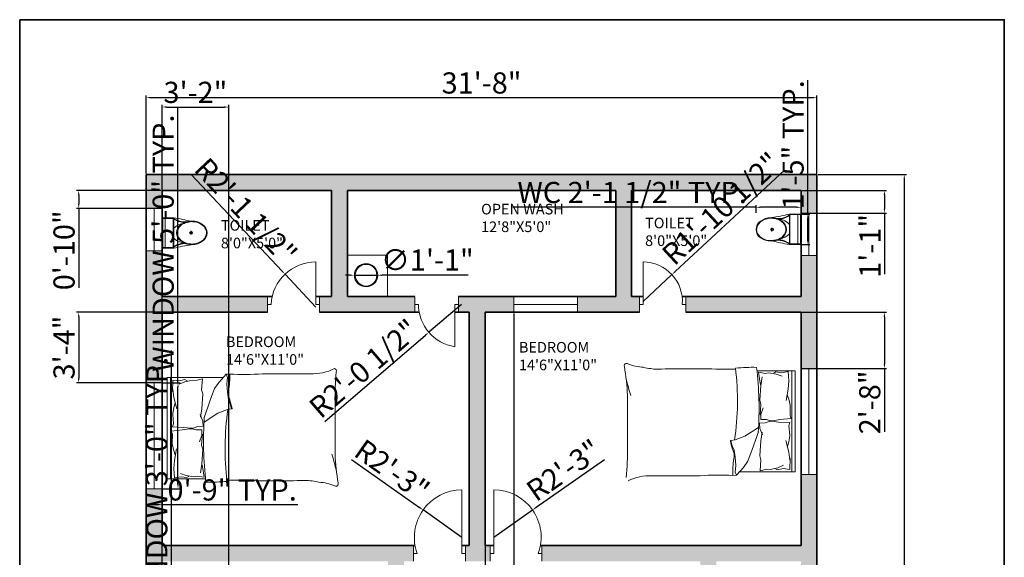
# Model space of a CAD drawing. Units: inches. Extents: x 995 to 1625, y 1005 to 1825.
# Tile 5 of 5: x 995 to 1553, y 1521 to 1825. Entities that reach past the tile are written whole.
import ezdxf

# ---------------------------------------------------------------- set-up
doc = ezdxf.new("R2010")
doc.units = ezdxf.units.IN
for name, color, linetype, lineweight in [('A-ANNO-DIMS', 2, 'Continuous', 18), ('A-ANNO-TTLB', 7, 'Continuous', 35), ('A-AREA-IDEN', 7, 'Continuous', 18), ('A-DOOR', 4, 'Continuous', 18), ('A-FLOR-FIXT', 9, 'Continuous', 18), ('A-FURN', 8, 'Continuous', 13), ('A-GLAZ', 3, 'Continuous', 18), ('A-WALL', 7, 'Continuous', 35)]:
    doc.layers.add(name, color=color, linetype=linetype, lineweight=lineweight)
doc.layers.add('A-WALL-PATT', color=251, linetype='Continuous', lineweight=13, true_color=0x636466)
doc.styles.get("Standard").update_dxf_attribs({"font": 'arial.ttf'})
doc.dimstyles.new('ISO-25', dxfattribs={"dimtxt": 12, "dimasz": 2.5, "dimexe": 1.25, "dimexo": 0.625, "dimtad": 1, "dimdec": 0, "dimlunit": 3, "dimtxsty": 'Standard', "dimcen": 2.5, "dimadec": 0, "dimazin": 0, "dimtfac": 1, "dimtdec": 0, "dimtmove": 0, "dimatfit": 3, "dimfxl": 1, "dimarcsym": 0})

# ---------------------------------------------------------------- blocks, each defined once
blk = doc.blocks.new('*D4')
at = {"layer": 'A-ANNO-DIMS', "color": 0, "lineweight": -2, "transparency": 16777216}
for p, q in [((1447.49, 1737.43), (1497.61, 1737.43)), ((1496.36, 1734.93), (1496.36, 1109.93)), ((1447.49, 1107.43), (1497.61, 1107.43))]:
    blk.add_line(p, q, dxfattribs=at)
at = {"layer": 'A-ANNO-DIMS', "color": 0, "transparency": 16777216}
for points in [[(1495.94, 1734.93), (1496.78, 1734.93), (1496.36, 1737.43)], [(1495.94, 1109.93), (1496.78, 1109.93), (1496.36, 1107.43)]]:
    blk.add_solid(points, dxfattribs=at)
at = {"layer": 'Defpoints', "color": 0, "transparency": 16777216}
for p in [(1446.87, 1737.43), (1446.87, 1107.43), (1496.36, 1107.43)]:
    blk.add_point(p, dxfattribs=at)
at = {"layer": 'A-ANNO-DIMS', "color": 0, "transparency": 16777216, "insert": (1489.61, 1422.43), "char_height": 12, "attachment_point": 5, "rotation": 90}
blk.add_mtext('52\'-6"', dxfattribs=at)
blk = doc.blocks.new('*D5')
at = {"layer": 'A-ANNO-DIMS', "color": 0, "lineweight": -2, "transparency": 16777216}
for p, q in [((1066.87, 1738.05), (1066.87, 1782.25)), ((1069.37, 1781), (1444.37, 1781)), ((1446.87, 1738.05), (1446.87, 1782.25))]:
    blk.add_line(p, q, dxfattribs=at)
at = {"layer": 'A-ANNO-DIMS', "color": 0, "transparency": 16777216}
for points in [[(1069.37, 1781.42), (1069.37, 1780.58), (1066.87, 1781)], [(1444.37, 1781.42), (1444.37, 1780.58), (1446.87, 1781)]]:
    blk.add_solid(points, dxfattribs=at)
at = {"layer": 'Defpoints', "color": 0, "transparency": 16777216}
for p in [(1446.87, 1781), (1066.87, 1737.43), (1446.87, 1737.43)]:
    blk.add_point(p, dxfattribs=at)
at = {"layer": 'A-ANNO-DIMS', "color": 0, "transparency": 16777216, "insert": (1256.87, 1787.76), "char_height": 12, "attachment_point": 5}
blk.add_mtext('31\'-8"', dxfattribs=at)
blk = doc.blocks.new('A$C31115884')
for p, q in [((258, 466), (258, 523)), ((283, 498), (223, 498)), ((0, 200), (0, 0)), ((520, 200), (0, 200)), ((10, 190), (10, 10)), ((510, 190), (10, 190)), ((510, 10), (510, 190)), ((520, 0), (520, 200)), ((510, 54), (0, 54)), ((10, 10), (510, 10)), ((0, 0), (520, 0))]:
    blk.add_line(p, q)
blk.add_circle((256, 496), 23.6)
for centre, radius, start, end in [((2778, -205), 2807, 165.4549, 171.7133), ((-295, 403), 365, 324.2091, 9.3499), ((-295, 403), 375, 324.2091, 9.3499), ((384, 406), 293, 190.2774, 224.1564), ((139, 406), 293, 315.8436, 2.6563), ((806, 403), 375, 179.2036, 215.7909), ((806, 403), 365, 170.6501, 215.7909), ((3237, 905), 2807, 188.2867, 194.5451)]:
    blk.add_arc(centre, radius, start, end)
blk.add_ellipse((256, 510), major_axis=(0, -261), ratio=0.772727)
blk.add_open_spline([(256, 259), (263, 259), (270, 260), (288, 262), (299, 265), (320, 273), (330, 278), (350, 291), (360, 299), (378, 316), (386, 326), (402, 347), (409, 358), (421, 383), (427, 395), (436, 422), (440, 436), (445, 465), (447, 480), (448, 509), (448, 524), (445, 553), (443, 568), (436, 596), (432, 610), (422, 636), (416, 649), (402, 672), (395, 683), (379, 703), (370, 712), (351, 728), (341, 735), (321, 746), (310, 751), (289, 757), (278, 759), (256, 761), (245, 761), (223, 757), (212, 754), (191, 746), (181, 741), (161, 728), (151, 720), (133, 703), (125, 693), (110, 672), (103, 660), (90, 636), (85, 623), (76, 596), (72, 582), (67, 553), (66, 538), (64, 509), (65, 494), (68, 465), (70, 450), (77, 422), (81, 408), (91, 382), (97, 370), (111, 346), (118, 335), (135, 316), (144, 307), (162, 291), (172, 284), (193, 273), (203, 269), (225, 262), (236, 260), (250, 259), (253, 259), (256, 259)], degree=3, knots=[0, 0, 0, 0, 0.110105, 0.110105, 0.285049, 0.285049, 0.459994, 0.459994, 0.634938, 0.634938, 0.809882, 0.809882, 0.984827, 0.984827, 1.159771, 1.159771, 1.334715, 1.334715, 1.50966, 1.50966, 1.684604, 1.684604, 1.859549, 1.859549, 2.034493, 2.034493, 2.209437, 2.209437, 2.384382, 2.384382, 2.559326, 2.559326, 2.73427, 2.73427, 2.909215, 2.909215, 3.084159, 3.084159, 3.259103, 3.259103, 3.434048, 3.434048, 3.608992, 3.608992, 3.783936, 3.783936, 3.958881, 3.958881, 4.133825, 4.133825, 4.30877, 4.30877, 4.483714, 4.483714, 4.658658, 4.658658, 4.833603, 4.833603, 5.008547, 5.008547, 5.183491, 5.183491, 5.358436, 5.358436, 5.53338, 5.53338, 5.708324, 5.708324, 5.883269, 5.883269, 6.058213, 6.058213, 6.233158, 6.233158, 6.283185, 6.283185, 6.283185, 6.283185])
blk = doc.blocks.new('WIN-24IN')
for p, q in [((0, 0), (0, -9)), ((24, -4.5), (24, 0)), ((24, 0), (24, -9)), ((0, -9), (0, -4.5)), ((0, -4.5), (24, -4.5))]:
    blk.add_line(p, q)
blk = doc.blocks.new('WIN-60IN')
for p, q in [((0, 0), (9, 0)), ((9, 0), (4.5, 0)), ((4.5, 0), (4.5, -60)), ((4.5, -60), (0, -60)), ((0, -60), (9, -60))]:
    blk.add_line(p, q)
blk = doc.blocks.new('WIN-36IN')
for p, q in [((0, 0), (9, 0)), ((9, 0), (4.5, 0)), ((4.5, 0), (4.5, -36)), ((4.5, -36), (0, -36)), ((0, -36), (9, -36))]:
    blk.add_line(p, q)
blk = doc.blocks.new('BED-DOUBLE')
for p, q in [((13.64, 59.31), (35.36, 59.31)), ((15.43, 52.35), (14.57, 58.46)), ((14.57, 58.46), (18.38, 57.77)), ((16.62, 55.83), (15.82, 50.99)), ((18.38, 57.77), (20.29, 58.11)), ((20.29, 58.11), (24.62, 57.42)), ((24.45, 58.63), (23.23, 57.94)), ((27.57, 58.11), (24.45, 58.63)), ((24.62, 57.42), (27.91, 56.21)), ((31.38, 58.81), (27.57, 58.11)), ((31.35, 58.8), (31.75, 53.67)), ((33.52, 59.31), (33.52, 2.02)), ((35.36, 59.31), (35.36, 2.02)), ((15.82, 50.99), (15.3, 42.59)), ((15.82, 50.99), (15.43, 52.35)), ((31.73, 53.54), (31.38, 48.96)), ((31.75, 53.67), (31.73, 53.54)), ((-59.65, 45.42), (-59.65, 15.91)), ((31.38, 48.96), (30.17, 42.37)), ((30.86, 45.67), (31.73, 43.24)), ((15.3, 42.59), (15.97, 40.24)), ((15.97, 40.24), (15.49, 34.09)), ((31.73, 43.24), (32.59, 39.77)), ((32.59, 39.39), (32.42, 34.06)), ((32.59, 39.77), (32.59, 39.39)), ((15.86, 34.58), (17.17, 38.35)), ((15.86, 31.63), (15.86, 34.58)), ((32.42, 34.06), (33.11, 32.33)), ((18.31, 29.75), (15.1, 29.55)), ((15.1, 29.55), (15.29, 26.61)), ((19.07, 31.63), (15.86, 31.63)), ((20.52, 30.58), (18.31, 29.75)), ((21.33, 30.94), (19.07, 31.63)), ((22.07, 30.68), (20.52, 30.58)), ((22.89, 30.94), (21.33, 30.94)), ((25.92, 30.23), (22.07, 30.68)), ((26.7, 31.63), (22.89, 30.94)), ((32.37, 29.94), (25.92, 30.23)), ((33.11, 32.33), (26.7, 31.63)), ((31.78, 28.16), (32.37, 29.94)), ((32.29, 22.85), (31.78, 28.16)), ((14.51, 27.2), (6.73, 22.18)), ((11, 14.75), (14.51, 24.75)), ((15.29, 26.61), (16.83, 22.93)), ((16.62, 24.44), (15.82, 19.6)), ((31.66, 18.96), (32.31, 22.47)), ((32.31, 22.47), (32.29, 22.85)), ((1.35, 20.13), (-1.06, 19.76)), ((-1.06, 19.76), (-0.32, 16.79)), ((-0.32, 16.79), (0.79, 14.38)), ((6.73, 22.18), (1.35, 20.13)), ((15.82, 19.6), (15.3, 11.2)), ((31.68, 13.23), (30.05, 19.72)), ((30.95, 16.48), (31.66, 18.96)), ((0.79, 14.38), (1.35, 10.29)), ((8.59, 8.07), (11, 14.75)), ((15.3, 11.2), (15.97, 8.85)), ((32.31, 8.67), (31.68, 13.23)), ((1.35, 10.29), (1.72, 5.65)), ((1.72, 5.65), (1.35, 1.94)), ((5.99, 4.54), (8.59, 8.07)), ((15.97, 8.85), (15.49, 2.7)), ((25.46, 4.36), (28.67, 5.78)), ((32.29, 3.4), (32.41, 9.88)), ((32.41, 9.88), (32.31, 8.67)), ((0, 0), (2.09, 0.1, 4.64)), ((1.35, 1.94), (2.09, 0.1)), ((2.09, 0.1), (5.99, 4.54)), ((35.36, 2.02), (3.45, 2.02)), ((15.49, 2.7), (19.25, 3.63)), ((19.25, 3.63), (21.17, 3.4)), ((21.17, 3.4), (25.46, 4.36)), ((25.36, 3.14), (24.1, 3.76)), ((28.44, 3.85), (25.36, 3.14)), ((32.29, 3.4), (28.44, 3.85))]:
    blk.add_line(p, q)
for centre, radius, start, end in [((-60.22, 62.17), 1.31, 56.1736, 203.4781), ((-205.42, 37.79), 145.97, 2.9958, 9.4091), ((-48.9, 89.44), 28.25, 247.9751, 266.652), ((-41.99, 95.72), 35.53, 256.0648, 268.9113), ((-25.32, -517.76), 578.22, 88.22771, 91.71854), ((-2.02, 264.05), 203.94, 268.4762, 271.0082), ((-152.05, 42.19), 154.68, 351.7845, 6.9006), ((11.26, -38.62), 99.87, 88.7218, 95.604), ((-182.9, 37.87), 197.77, 356.0865, 6.7821), ((63.78, 84.12), 127.63, 193.3832, 197.7053), ((-1.14, 19.55), 0.221, 70.2464, 181.1377), ((33.58, 26.13), 35.55, 190.6617, 199.8806), ((-219.13, 14.14), 159.5, 354.4998, 0.6351), ((-6.68, 11.03), 7.46, 348.6608, 23.7384), ((43.33, 1.94), 43.38, 169.8763, 182.5657), ((-8.18, -155.03), 155.25, 86.9791, 93.8365), ((-46.97, -27.83), 27.65, 87.4714, 116.4681), ((-45.95, 5468.82), 5469.02, 270.00217, 270.28689)]:
    blk.add_arc(centre, radius, start, end)
blk = doc.blocks.new('*D14')
at = {"layer": 'A-ANNO-DIMS', "color": 0, "lineweight": -2, "transparency": 16777216}
for p, q in [((1081.27, 1482.29), (1081.27, 1637.89)), ((1076.49, 1482.29), (1082.52, 1482.29)), ((1081.27, 1448.79), (1081.27, 1479.79)), ((1076.49, 1446.29), (1082.52, 1446.29))]:
    blk.add_line(p, q, dxfattribs=at)
at = {"layer": 'A-ANNO-DIMS', "color": 0, "transparency": 16777216}
for points in [[(1080.85, 1479.79), (1081.68, 1479.79), (1081.27, 1482.29)], [(1080.85, 1448.79), (1081.68, 1448.79), (1081.27, 1446.29)]]:
    blk.add_solid(points, dxfattribs=at)
at = {"layer": 'Defpoints', "color": 0, "transparency": 16777216}
for p in [(1075.87, 1482.29), (1081.27, 1482.29), (1075.87, 1446.29)]:
    blk.add_point(p, dxfattribs=at)
at = {"layer": 'A-ANNO-DIMS', "color": 0, "transparency": 16777216, "insert": (1074.43, 1561.34), "char_height": 12, "attachment_point": 5, "rotation": 90}
blk.add_mtext('WINDOW 3\'-0" TYP.', dxfattribs=at)
blk = doc.blocks.new('*D16')
at = {"layer": 'A-ANNO-DIMS', "color": 0, "lineweight": -2, "transparency": 16777216}
for p, q in [((1084.87, 1619.54), (1084.87, 1775.14)), ((1076.49, 1619.54), (1086.12, 1619.54)), ((1084.87, 1562.04), (1084.87, 1617.04)), ((1076.49, 1559.54), (1086.12, 1559.54))]:
    blk.add_line(p, q, dxfattribs=at)
at = {"layer": 'A-ANNO-DIMS', "color": 0, "transparency": 16777216}
for points in [[(1084.45, 1617.04), (1085.28, 1617.04), (1084.87, 1619.54)], [(1084.45, 1562.04), (1085.28, 1562.04), (1084.87, 1559.54)]]:
    blk.add_solid(points, dxfattribs=at)
at = {"layer": 'Defpoints', "color": 0, "transparency": 16777216}
for p in [(1075.87, 1619.54), (1084.87, 1619.54), (1075.87, 1559.54)]:
    blk.add_point(p, dxfattribs=at)
at = {"layer": 'A-ANNO-DIMS', "color": 0, "transparency": 16777216, "insert": (1078.03, 1698.59), "char_height": 12, "attachment_point": 5, "rotation": 90}
blk.add_mtext('WINDOW 5\'-0" TYP.', dxfattribs=at)
blk = doc.blocks.new('*D17')
at = {"layer": 'A-ANNO-DIMS', "color": 0, "lineweight": -2, "transparency": 16777216}
for p, q in [((1066.87, 1558.91), (1066.87, 1549.29)), ((1075.87, 1558.91), (1075.87, 1549.29)), ((1069.37, 1550.54), (1073.37, 1550.54)), ((1075.87, 1550.54), (1152.76, 1550.54))]:
    blk.add_line(p, q, dxfattribs=at)
at = {"layer": 'A-ANNO-DIMS', "color": 0, "transparency": 16777216}
for points in [[(1069.37, 1550.96), (1069.37, 1550.12), (1066.87, 1550.54)], [(1073.37, 1550.96), (1073.37, 1550.12), (1075.87, 1550.54)]]:
    blk.add_solid(points, dxfattribs=at)
at = {"layer": 'Defpoints', "color": 0, "transparency": 16777216}
for p in [(1066.87, 1559.54), (1075.87, 1559.54), (1075.87, 1550.54)]:
    blk.add_point(p, dxfattribs=at)
at = {"layer": 'A-ANNO-DIMS', "color": 0, "transparency": 16777216, "insert": (1115.56, 1557.29), "char_height": 12, "attachment_point": 5}
blk.add_mtext('0\'-9" TYP.', dxfattribs=at)
blk = doc.blocks.new('*D22')
at = {"layer": 'A-ANNO-DIMS', "color": 0, "lineweight": -2, "transparency": 16777216}
for p, q in [((1412.39, 1718.9), (1274.45, 1718.9)), ((1412.39, 1715.71), (1412.39, 1720.15)), ((1435.37, 1718.9), (1414.89, 1718.9)), ((1437.87, 1715.71), (1437.87, 1720.15))]:
    blk.add_line(p, q, dxfattribs=at)
at = {"layer": 'A-ANNO-DIMS', "color": 0, "transparency": 16777216}
for points in [[(1414.89, 1719.32), (1414.89, 1718.49), (1412.39, 1718.9)], [(1435.37, 1719.32), (1435.37, 1718.49), (1437.87, 1718.9)]]:
    blk.add_solid(points, dxfattribs=at)
at = {"layer": 'Defpoints', "color": 0, "transparency": 16777216}
for p in [(1412.39, 1718.9), (1412.39, 1715.08), (1437.87, 1715.08)]:
    blk.add_point(p, dxfattribs=at)
at = {"layer": 'A-ANNO-DIMS', "color": 0, "transparency": 16777216, "insert": (1342.17, 1725.73), "char_height": 12, "attachment_point": 5}
blk.add_mtext('WC 2\'-1 1/2" TYP.', dxfattribs=at)
blk = doc.blocks.new('*D23')
at = {"layer": 'A-ANNO-DIMS', "color": 0, "lineweight": -2, "transparency": 16777216}
for p, q in [((1441.69, 1715.08), (1441.69, 1790.85)), ((1438.49, 1715.08), (1442.94, 1715.08)), ((1441.69, 1700.39), (1441.69, 1712.58)), ((1438.49, 1697.89), (1442.94, 1697.89))]:
    blk.add_line(p, q, dxfattribs=at)
at = {"layer": 'A-ANNO-DIMS', "color": 0, "transparency": 16777216}
for points in [[(1441.27, 1712.58), (1442.1, 1712.58), (1441.69, 1715.08)], [(1441.27, 1700.39), (1442.1, 1700.39), (1441.69, 1697.89)]]:
    blk.add_solid(points, dxfattribs=at)
at = {"layer": 'Defpoints', "color": 0, "transparency": 16777216}
for p in [(1437.87, 1715.08), (1441.69, 1715.08), (1437.87, 1697.89)]:
    blk.add_point(p, dxfattribs=at)
at = {"layer": 'A-ANNO-DIMS', "color": 0, "transparency": 16777216, "insert": (1434.94, 1754.21), "char_height": 12, "attachment_point": 5, "rotation": 90}
blk.add_mtext('1\'-5" TYP.', dxfattribs=at)
blk = doc.blocks.new('*D27')
at = {"layer": 'A-ANNO-DIMS', "color": 0, "lineweight": -2, "transparency": 16777216}
for p, q in [((1075.87, 1339.51), (1075.87, 1776.93)), ((1078.37, 1775.68), (1111.14, 1775.68)), ((1113.64, 1339.51), (1113.64, 1776.93))]:
    blk.add_line(p, q, dxfattribs=at)
at = {"layer": 'A-ANNO-DIMS', "color": 0, "transparency": 16777216}
for points in [[(1078.37, 1776.09), (1078.37, 1775.26), (1075.87, 1775.68)], [(1111.14, 1776.09), (1111.14, 1775.26), (1113.64, 1775.68)]]:
    blk.add_solid(points, dxfattribs=at)
at = {"layer": 'Defpoints', "color": 0, "transparency": 16777216}
for p in [(1113.64, 1775.68), (1075.87, 1338.88), (1113.64, 1338.88)]:
    blk.add_point(p, dxfattribs=at)
at = {"layer": 'A-ANNO-DIMS', "color": 0, "transparency": 16777216, "insert": (1094.75, 1782.43), "char_height": 12, "attachment_point": 5}
blk.add_mtext('3\'-2"', dxfattribs=at)
blk = doc.blocks.new('*D33')
at = {"layer": 'A-ANNO-DIMS', "color": 0, "lineweight": -2, "transparency": 16777216}
for p, q in [((1075.24, 1728.43), (1027.37, 1728.43)), ((1028.62, 1725.93), (1028.62, 1720.78)), ((1075.24, 1718.28), (1027.37, 1718.28)), ((1028.62, 1718.28), (1028.62, 1673.31))]:
    blk.add_line(p, q, dxfattribs=at)
at = {"layer": 'A-ANNO-DIMS', "color": 0, "transparency": 16777216}
for points in [[(1028.2, 1725.93), (1029.03, 1725.93), (1028.62, 1728.43)], [(1028.2, 1720.78), (1029.03, 1720.78), (1028.62, 1718.28)]]:
    blk.add_solid(points, dxfattribs=at)
at = {"layer": 'Defpoints', "color": 0, "transparency": 16777216}
for p in [(1075.87, 1728.43), (1028.62, 1718.28), (1075.87, 1718.28)]:
    blk.add_point(p, dxfattribs=at)
at = {"layer": 'A-ANNO-DIMS', "color": 0, "transparency": 16777216, "insert": (1021.86, 1694.54), "char_height": 12, "attachment_point": 5, "rotation": 90}
blk.add_mtext('0\'-10"', dxfattribs=at)
blk = doc.blocks.new('*D34')
at = {"layer": 'A-ANNO-DIMS', "color": 0, "lineweight": -2, "transparency": 16777216}
for p, q in [((1438.49, 1728.43), (1486.37, 1728.43)), ((1485.12, 1725.93), (1485.12, 1718.06)), ((1438.49, 1715.56), (1486.37, 1715.56)), ((1485.12, 1715.56), (1485.12, 1681.04))]:
    blk.add_line(p, q, dxfattribs=at)
at = {"layer": 'A-ANNO-DIMS', "color": 0, "transparency": 16777216}
for points in [[(1484.7, 1725.93), (1485.53, 1725.93), (1485.12, 1728.43)], [(1484.7, 1718.06), (1485.53, 1718.06), (1485.12, 1715.56)]]:
    blk.add_solid(points, dxfattribs=at)
at = {"layer": 'Defpoints', "color": 0, "transparency": 16777216}
for p in [(1437.87, 1728.43), (1437.87, 1715.56), (1485.12, 1715.56)]:
    blk.add_point(p, dxfattribs=at)
at = {"layer": 'A-ANNO-DIMS', "color": 0, "transparency": 16777216, "insert": (1478.47, 1697.05), "char_height": 12, "attachment_point": 5, "rotation": 90}
blk.add_mtext('1\'-1"', dxfattribs=at)
blk = doc.blocks.new('*D35')
at = {"layer": 'A-ANNO-DIMS', "color": 0, "lineweight": -2, "transparency": 16777216}
for p, q in [((1075.24, 1659.43), (1027.37, 1659.43)), ((1028.62, 1656.93), (1028.62, 1622.04)), ((1075.24, 1619.54), (1027.37, 1619.54))]:
    blk.add_line(p, q, dxfattribs=at)
at = {"layer": 'A-ANNO-DIMS', "color": 0, "transparency": 16777216}
for points in [[(1028.2, 1656.93), (1029.03, 1656.93), (1028.62, 1659.43)], [(1028.2, 1622.04), (1029.03, 1622.04), (1028.62, 1619.54)]]:
    blk.add_solid(points, dxfattribs=at)
at = {"layer": 'Defpoints', "color": 0, "transparency": 16777216}
for p in [(1075.87, 1659.43), (1028.62, 1619.54), (1075.87, 1619.54)]:
    blk.add_point(p, dxfattribs=at)
at = {"layer": 'A-ANNO-DIMS', "color": 0, "transparency": 16777216, "insert": (1021.86, 1639.48), "char_height": 12, "attachment_point": 5, "rotation": 90}
blk.add_mtext('3\'-4"', dxfattribs=at)
blk = doc.blocks.new('*D36')
at = {"layer": 'A-ANNO-DIMS', "color": 0, "lineweight": -2, "transparency": 16777216}
for p, q in [((1438.49, 1659.43), (1486.37, 1659.43)), ((1485.12, 1656.93), (1485.12, 1630.08)), ((1438.49, 1627.58), (1486.37, 1627.58)), ((1485.12, 1627.58), (1485.12, 1591.72))]:
    blk.add_line(p, q, dxfattribs=at)
at = {"layer": 'A-ANNO-DIMS', "color": 0, "transparency": 16777216}
for points in [[(1484.7, 1656.93), (1485.53, 1656.93), (1485.12, 1659.43)], [(1484.7, 1630.08), (1485.53, 1630.08), (1485.12, 1627.58)]]:
    blk.add_solid(points, dxfattribs=at)
at = {"layer": 'Defpoints', "color": 0, "transparency": 16777216}
for p in [(1437.87, 1659.43), (1437.87, 1627.58), (1485.12, 1627.58)]:
    blk.add_point(p, dxfattribs=at)
at = {"layer": 'A-ANNO-DIMS', "color": 0, "transparency": 16777216, "insert": (1478.36, 1608.4), "char_height": 12, "attachment_point": 5, "rotation": 90}
blk.add_mtext('2\'-8"', dxfattribs=at)
blk = doc.blocks.new('*D37')
at = {"layer": 'A-ANNO-DIMS', "color": 0, "lineweight": -2, "transparency": 16777216}
for p, q in [((1258.87, 1658.8), (1258.87, 1015.27)), ((1275.16, 1658.8), (1275.16, 1015.27)), ((1261.37, 1016.52), (1272.66, 1016.52)), ((1275.16, 1016.52), (1337.64, 1016.52))]:
    blk.add_line(p, q, dxfattribs=at)
at = {"layer": 'A-ANNO-DIMS', "color": 0, "transparency": 16777216}
for points in [[(1261.37, 1016.93), (1261.37, 1016.1), (1258.87, 1016.52)], [(1272.66, 1016.93), (1272.66, 1016.1), (1275.16, 1016.52)]]:
    blk.add_solid(points, dxfattribs=at)
at = {"layer": 'Defpoints', "color": 0, "transparency": 16777216}
for p in [(1258.87, 1659.43), (1275.16, 1659.43), (1275.16, 1016.52)]:
    blk.add_point(p, dxfattribs=at)
at = {"layer": 'A-ANNO-DIMS', "color": 0, "transparency": 16777216, "insert": (1307.65, 1023.35), "char_height": 12, "attachment_point": 5}
blk.add_mtext('1\'-4 1/2"', dxfattribs=at)
blk = doc.blocks.new('*D43')
at = {"layer": 'A-ANNO-DIMS', "color": 0, "lineweight": -2, "transparency": 16777216}
for p, q in [((1182.33, 1680.43), (1179.83, 1680.43)), ((1184.83, 1680.43), (1198.05, 1680.43)), ((1249.25, 1680.42), (1200.55, 1680.43))]:
    blk.add_line(p, q, dxfattribs=at)
at = {"layer": 'A-ANNO-DIMS', "color": 0, "transparency": 16777216}
for points in [[(1182.33, 1680.84), (1182.33, 1680.01), (1184.83, 1680.43)], [(1200.55, 1680.84), (1200.55, 1680.01), (1198.05, 1680.43)]]:
    blk.add_solid(points, dxfattribs=at)
at = {"layer": 'Defpoints', "color": 0, "transparency": 16777216}
for p in [(1184.83, 1680.43), (1198.05, 1680.43)]:
    blk.add_point(p, dxfattribs=at)
at = {"layer": 'A-ANNO-DIMS', "color": 0, "transparency": 16777216, "insert": (1226.15, 1687.51), "char_height": 12, "attachment_point": 5, "rotation": 359.9975}
blk.add_mtext('∅1\'-1"', dxfattribs=at)
blk = doc.blocks.new('*D46')
at = {"layer": 'A-ANNO-DIMS', "color": 0, "lineweight": -2, "transparency": 16777216}
for p, q in [((1183.17, 1576.14), (1221.67, 1548.95)), ((1245.75, 1531.95), (1223.71, 1547.51))]:
    blk.add_line(p, q, dxfattribs=at)
at = {"layer": 'A-ANNO-DIMS', "color": 0, "transparency": 16777216}
blk.add_solid([(1221.91, 1549.29), (1221.43, 1548.61), (1223.71, 1547.51)], dxfattribs=at)
at = {"layer": 'Defpoints', "color": 0, "transparency": 16777216}
for p in [(1223.71, 1547.51), (1245.75, 1531.95)]:
    blk.add_point(p, dxfattribs=at)
at = {"layer": 'A-ANNO-DIMS', "color": 0, "transparency": 16777216, "insert": (1205.29, 1568.79), "char_height": 12, "attachment_point": 5, "rotation": 324.773}
blk.add_mtext('R2\'-3"', dxfattribs=at)
blk = doc.blocks.new('*D47')
at = {"layer": 'A-ANNO-DIMS', "color": 0, "lineweight": -2, "transparency": 16777216}
for p, q in [((1326.45, 1575.96), (1287.84, 1548.92)), ((1263.81, 1532.1), (1285.79, 1547.49))]:
    blk.add_line(p, q, dxfattribs=at)
at = {"layer": 'A-ANNO-DIMS', "color": 0, "transparency": 16777216}
blk.add_solid([(1287.6, 1549.26), (1288.08, 1548.58), (1285.79, 1547.49)], dxfattribs=at)
at = {"layer": 'Defpoints', "color": 0, "transparency": 16777216}
for p in [(1285.79, 1547.49), (1263.81, 1532.1)]:
    blk.add_point(p, dxfattribs=at)
at = {"layer": 'A-ANNO-DIMS', "color": 0, "transparency": 16777216, "insert": (1304.29, 1568.69), "char_height": 12, "attachment_point": 5, "rotation": 35.0018}
blk.add_mtext('R2\'-3"', dxfattribs=at)
blk = doc.blocks.new('*D48')
at = {"layer": 'A-ANNO-DIMS', "color": 0, "lineweight": -2, "transparency": 16777216}
for p, q in [((1092.34, 1737.46), (1143.84, 1682.8)), ((1163.05, 1662.41), (1145.56, 1680.98))]:
    blk.add_line(p, q, dxfattribs=at)
at = {"layer": 'A-ANNO-DIMS', "color": 0, "transparency": 16777216}
blk.add_solid([(1144.14, 1683.09), (1143.54, 1682.52), (1145.56, 1680.98)], dxfattribs=at)
at = {"layer": 'Defpoints', "color": 0, "transparency": 16777216}
for p in [(1145.56, 1680.98), (1163.05, 1662.41)]:
    blk.add_point(p, dxfattribs=at)
at = {"layer": 'A-ANNO-DIMS', "color": 0, "transparency": 16777216, "insert": (1122.21, 1715.72), "char_height": 12, "attachment_point": 5, "rotation": 313.295}
blk.add_mtext('R2\'-1 1/2"', dxfattribs=at)
blk = doc.blocks.new('*D49')
at = {"layer": 'A-ANNO-DIMS', "color": 0, "lineweight": -2, "transparency": 16777216}
for p, q in [((1245.41, 1663.93), (1226.99, 1648.11)), ((1168.12, 1597.55), (1225.09, 1646.48))]:
    blk.add_line(p, q, dxfattribs=at)
at = {"layer": 'A-ANNO-DIMS', "color": 0, "transparency": 16777216}
blk.add_solid([(1224.82, 1646.8), (1225.36, 1646.16), (1226.99, 1648.11)], dxfattribs=at)
at = {"layer": 'Defpoints', "color": 0, "transparency": 16777216}
for p in [(1245.41, 1663.93), (1226.99, 1648.11)]:
    blk.add_point(p, dxfattribs=at)
at = {"layer": 'A-ANNO-DIMS', "color": 0, "transparency": 16777216, "insert": (1191.21, 1626.38), "char_height": 12, "attachment_point": 5, "rotation": 40.656}
blk.add_mtext('R2\'-0 1/2"', dxfattribs=at)
blk = doc.blocks.new('*D52')
at = {"layer": 'A-ANNO-DIMS', "color": 0, "lineweight": -2, "transparency": 16777216}
for p, q in [((1428.46, 1739.87), (1366.55, 1682.48)), ((1348.35, 1665.62), (1364.72, 1680.78))]:
    blk.add_line(p, q, dxfattribs=at)
at = {"layer": 'A-ANNO-DIMS', "color": 0, "transparency": 16777216}
blk.add_solid([(1366.27, 1682.79), (1366.83, 1682.18), (1364.72, 1680.78)], dxfattribs=at)
at = {"layer": 'Defpoints', "color": 0, "transparency": 16777216}
for p in [(1364.72, 1680.78), (1348.35, 1665.62)]:
    blk.add_point(p, dxfattribs=at)
at = {"layer": 'A-ANNO-DIMS', "color": 0, "transparency": 16777216, "insert": (1393.78, 1717.03), "char_height": 12, "attachment_point": 5, "rotation": 42.8258}
blk.add_mtext('R1\'-10 1/2"', dxfattribs=at)

msp = doc.modelspace()

# ---------------------------------------------------------------- hatches: boundary and pattern name
at = {"layer": 'A-WALL-PATT'}
h = msp.add_hatch(color=256, dxfattribs=at)
h.dxf.hatch_style = 1
h.paths.add_polyline_path([(1446.87, 1737.43), (1066.87, 1737.43), (1066.87, 1718.28), (1075.87, 1718.28), (1075.87, 1728.43), (1171.87, 1728.43), (1171.87, 1668.43), (1165.05, 1668.43), (1165.05, 1659.43), (1219.13, 1659.43), (1219.13, 1663.93), (1219.13, 1668.43), (1180.87, 1668.43), (1180.87, 1691.88), (1180.87, 1728.43), (1249.87, 1728.43), (1258.87, 1728.43), (1332.87, 1728.43), (1332.87, 1668.43), (1311.16, 1668.43), (1311.16, 1659.43), (1346.35, 1659.43), (1346.35, 1663.93), (1346.35, 1668.43), (1341.87, 1668.43), (1341.87, 1728.43), (1437.87, 1728.43), (1437.87, 1715.56), (1446.87, 1715.56)])
h.paths.add_polyline_path([(1135.58, 1663.93), (1135.58, 1668.43), (1075.87, 1668.43), (1075.87, 1694.28), (1066.87, 1694.28), (1066.87, 1619.54), (1075.87, 1619.54), (1075.87, 1659.43), (1135.58, 1659.43)])
h.paths.add_polyline_path([(1258.87, 1659.43), (1275.16, 1659.43), (1275.16, 1663.93), (1275.16, 1668.43), (1258.87, 1668.43), (1249.87, 1668.43), (1243.74, 1668.43), (1243.74, 1659.43), (1249.87, 1659.43), (1249.87, 1527.43), (1247.75, 1527.43), (1247.75, 1518.43), (1261.81, 1518.43), (1261.81, 1527.43), (1258.87, 1527.43)])
h.paths.add_polyline_path([(1446.87, 1691.56), (1437.87, 1691.56), (1437.87, 1668.43), (1372.6, 1668.43), (1372.6, 1659.43), (1437.87, 1659.43), (1437.87, 1627.58), (1446.87, 1627.58)])
h.paths.add_polyline_path([(1446.87, 1567.58), (1437.87, 1567.58), (1437.87, 1527.43), (1291.03, 1527.43), (1291.03, 1518.43), (1380.87, 1518.43), (1380.87, 1508.92), (1389.87, 1508.92), (1389.87, 1518.43), (1437.87, 1518.43), (1437.87, 1501.62), (1446.87, 1501.62)])
h.paths.add_polyline_path([(1446.87, 1477.62), (1437.87, 1477.62), (1437.87, 1429.75), (1446.87, 1429.75)])
h.paths.add_polyline_path([(1389.87, 1441.43), (1437.87, 1441.43), (1437.87, 1450.43), (1389.87, 1450.43), (1389.87, 1481.88), (1385.37, 1481.88), (1380.87, 1481.88), (1380.87, 1385.88), (1389.87, 1385.88)])
h.paths.add_polyline_path([(1446.87, 1405.75), (1437.87, 1405.75), (1437.87, 1350.43), (1427.33, 1350.43), (1389.87, 1350.43), (1389.87, 1359.9), (1380.87, 1359.9), (1380.87, 1350.43), (1324.85, 1350.43), (1324.85, 1341.43), (1437.87, 1341.43), (1437.87, 1303.84), (1446.87, 1303.84)])
h.paths.add_polyline_path([(1311.82, 1209.43), (1281.87, 1209.43), (1281.87, 1341.43), (1291.29, 1341.43), (1291.29, 1345.93), (1291.29, 1350.43), (1244.83, 1350.43), (1244.83, 1341.43), (1272.87, 1341.43), (1272.87, 1185.43), (1268.73, 1185.43), (1268.73, 1176.43), (1272.87, 1176.43), (1281.87, 1176.43), (1281.87, 1200.43), (1311.82, 1200.43), (1311.82, 1204.93)])
h.paths.add_polyline_path([(1446.87, 1243.84), (1437.87, 1243.84), (1437.87, 1209.43), (1371.82, 1209.43), (1371.82, 1200.43), (1437.87, 1200.43), (1437.87, 1107.43), (1446.87, 1107.43)])
h.paths.add_polyline_path([(1212.11, 1185.43), (1207.85, 1185.43), (1207.85, 1176.43), (1212.11, 1176.43)], flags=17)
h.paths.add_polyline_path([(1244.73, 1185.43), (1240.24, 1185.43), (1240.24, 1176.43), (1244.73, 1176.43), (1244.73, 1180.93)])
h.paths.add_polyline_path([(1183.85, 1180.93), (1183.85, 1185.43), (1180.87, 1185.43), (1180.87, 1191.84), (1171.87, 1191.84), (1171.87, 1176.43), (1180.87, 1176.43), (1183.85, 1176.43)], flags=17)
h.paths.add_polyline_path([(1180.87, 1341.43), (1198.57, 1341.43), (1198.57, 1350.43), (1180.87, 1350.43), (1180.87, 1354.13), (1176.37, 1354.13), (1171.87, 1354.13), (1171.87, 1341.43), (1171.87, 1219.68), (1180.87, 1219.68)], flags=17)
h.paths.add_polyline_path([(1075.87, 1391.93), (1171.87, 1391.93), (1171.87, 1389.24), (1180.87, 1389.24), (1180.87, 1391.93), (1212.87, 1391.93), (1212.87, 1431.83), (1203.87, 1431.83), (1203.87, 1400.93), (1075.87, 1400.93), (1075.87, 1446.29), (1066.87, 1446.29), (1066.87, 1107.43), (1075.87, 1107.43)])
h.paths.add_polyline_path([(1218.33, 1527.43), (1075.87, 1527.43), (1075.87, 1559.54), (1066.87, 1559.54), (1066.87, 1482.29), (1075.87, 1482.29), (1075.87, 1518.43), (1203.87, 1518.43), (1203.87, 1493.65), (1212.87, 1493.65), (1212.87, 1518.43), (1218.33, 1518.43), (1218.33, 1522.93)])
h.paths.add_polyline_path([(1297.68, 1457.37), (1297.68, 1425.03), (1310.04, 1425.03), (1310.04, 1457.37)], flags=9)
h.paths.add_polyline_path([(1154.86, 1054.62), (1346.22, 1054.62), (1346.22, 1079.35), (1154.86, 1079.35)], flags=9)
h.paths.add_polyline_path([(1237.85, 1265.85), (1262.06, 1265.85), (1262.06, 1288.24), (1237.85, 1288.24)], flags=9)
h.paths.add_polyline_path([(1331.39, 1305.41), (1378, 1305.41), (1378, 1327.8), (1331.39, 1327.8)], flags=25)
h.paths.add_polyline_path([(1395.38, 1378.18), (1431.86, 1378.18), (1431.86, 1400.57), (1395.38, 1400.57)], flags=25)
h.paths.add_polyline_path([(1406.34, 1460.18), (1434.48, 1460.18), (1434.48, 1472.55), (1406.34, 1472.55)], flags=25)
h.paths.add_polyline_path([(1134.66, 1454.9), (1180.38, 1454.9), (1180.38, 1477.29), (1134.66, 1477.29)], flags=9)
h.paths.add_polyline_path([(1109.63, 1626.32), (1156.23, 1626.32), (1156.23, 1648.71), (1109.63, 1648.71)], flags=9)
h.paths.add_polyline_path([(1275.64, 1623.22), (1322.25, 1623.22), (1322.25, 1645.61), (1275.64, 1645.61)], flags=9)
h.paths.add_polyline_path([(1347.7, 1693.6), (1384.09, 1693.6), (1384.09, 1715.99), (1347.7, 1715.99)], flags=25)
h.paths.add_polyline_path([(1254.21, 1701.46), (1308.94, 1701.46), (1308.94, 1723.85), (1254.21, 1723.85)], flags=25)
h.paths.add_polyline_path([(1107.35, 1692.25), (1143.74, 1692.25), (1143.74, 1714.64), (1107.35, 1714.64)], flags=25)

# ---------------------------------------------------------------- linework, layer by layer
at = {"layer": 'A-ANNO-TTLB'}
msp.add_lwpolyline([(995.18, 1825.14), (1553.05, 1825.14), (1553.05, 1020.2), (995.18, 1020.2)], close=True, dxfattribs=at)
at = {"layer": 'A-DOOR'}
for p, q in [((1163.05, 1663.93), (1163.05, 1687.93)), ((1348.35, 1663.93), (1348.35, 1687.93)), ((1135.58, 1668.43), (1135.58, 1659.43)), ((1165.05, 1668.43), (1165.05, 1659.43)), ((1219.13, 1668.43), (1219.13, 1659.43)), ((1243.74, 1668.43), (1243.74, 1659.43)), ((1346.35, 1668.43), (1346.35, 1659.43)), ((1372.6, 1668.43), (1372.6, 1659.43)), ((1135.58, 1659.43), (1135.58, 1663.93)), ((1135.58, 1663.93), (1137.58, 1663.93)), ((1165.05, 1663.93), (1163.05, 1663.93)), ((1165.05, 1659.43), (1165.05, 1663.93)), ((1219.13, 1659.43), (1219.13, 1663.93)), ((1219.13, 1663.93), (1221.13, 1663.93)), ((1243.74, 1663.93), (1241.74, 1663.93)), ((1241.74, 1663.93), (1241.74, 1639.93)), ((1243.74, 1659.43), (1243.74, 1663.93)), ((1346.35, 1659.43), (1346.35, 1663.93)), ((1346.35, 1663.93), (1348.35, 1663.93)), ((1372.6, 1663.93), (1370.6, 1663.93)), ((1372.6, 1659.43), (1372.6, 1663.93)), ((1245.75, 1522.93), (1245.75, 1558.93)), ((1263.81, 1522.93), (1263.81, 1558.93)), ((1218.33, 1527.43), (1218.33, 1518.43)), ((1247.75, 1527.43), (1247.75, 1518.43)), ((1261.81, 1527.43), (1261.81, 1518.43)), ((1291.03, 1527.43), (1291.03, 1518.43)), ((1218.33, 1518.43), (1218.33, 1522.93)), ((1218.33, 1522.93), (1220.33, 1522.93)), ((1247.75, 1522.93), (1245.75, 1522.93)), ((1261.81, 1522.93), (1263.81, 1522.93)), ((1291.03, 1522.93), (1289.03, 1522.93)), ((1291.03, 1518.43), (1291.03, 1522.93))]:
    msp.add_line(p, q, dxfattribs=at)
for centre, radius, start, end in [((1163.05, 1662.41), 25.52, 90, 176.592), ((1348.35, 1665.62), 22.31, 355.6533, 90), ((1245.41, 1663.93), 24.28, 180, 261.3119), ((1245.75, 1531.95), 26.97, 90, 199.5471), ((1263.81, 1532.1), 26.83, 340.006, 90)]:
    msp.add_arc(centre, radius, start, end, dxfattribs=at)
at = {"layer": 'A-FLOR-FIXT'}
msp.add_lwpolyline([(1180.87, 1691.88), (1203.55, 1691.88), (1203.55, 1668.43), (1180.87, 1668.43)], close=True, dxfattribs=at)
for radius in [6.61, 6.11]:
    msp.add_circle((1191.44, 1680.43), radius, dxfattribs=at)
at = {"layer": 'A-FURN'}
msp.add_arc((1173.39, 1626.2), 1.32, 332.6588, 86.02, dxfattribs=at)
at = {"layer": 'A-WALL'}
for p, q in [((1066.87, 1737.43), (1066.87, 1107.43)), ((1066.87, 1737.43), (1066.87, 1107.43)), ((1066.87, 1737.43), (1066.87, 1107.43)), ((1066.87, 1737.43), (1446.87, 1737.43)), ((1446.87, 1737.43), (1446.87, 1107.43)), ((1075.87, 1728.43), (1171.87, 1728.43)), ((1075.87, 1728.43), (1075.87, 1668.43)), ((1171.87, 1728.43), (1171.87, 1668.43)), ((1180.87, 1728.43), (1180.87, 1668.43)), ((1180.87, 1728.43), (1249.87, 1728.43)), ((1249.87, 1728.43), (1258.87, 1728.43)), ((1258.87, 1728.43), (1332.87, 1728.43)), ((1332.87, 1728.43), (1332.87, 1668.43)), ((1341.87, 1728.43), (1341.87, 1668.43)), ((1341.87, 1728.43), (1437.87, 1728.43)), ((1437.87, 1728.43), (1437.87, 1668.43)), ((1075.87, 1668.43), (1138.26, 1668.43)), ((1163.05, 1668.43), (1171.87, 1668.43)), ((1180.87, 1668.43), (1219.13, 1668.43)), ((1243.74, 1668.43), (1249.87, 1668.43)), ((1258.87, 1668.43), (1249.87, 1668.43)), ((1258.87, 1668.43), (1332.87, 1668.43)), ((1341.87, 1668.43), (1348.35, 1668.43)), ((1370.48, 1668.43), (1437.87, 1668.43)), ((1075.87, 1659.43), (1135.58, 1659.43)), ((1075.87, 1659.43), (1075.87, 1527.43)), ((1165.05, 1659.43), (1221.55, 1659.43)), ((1241.74, 1659.43), (1249.87, 1659.43)), ((1249.87, 1659.43), (1249.87, 1527.43)), ((1258.87, 1659.43), (1258.87, 1527.43)), ((1258.87, 1659.43), (1346.35, 1659.43)), ((1372.6, 1659.43), (1437.87, 1659.43)), ((1437.87, 1659.43), (1437.87, 1527.43)), ((1075.87, 1527.43), (1219.15, 1527.43)), ((1245.75, 1527.43), (1249.87, 1527.43)), ((1258.87, 1527.43), (1263.81, 1527.43)), ((1290.23, 1527.43), (1437.87, 1527.43))]:
    msp.add_line(p, q, dxfattribs=at)

# ---------------------------------------------------------------- block references
at = {"layer": 'A-FLOR-FIXT', "xscale": 0.0330640103915726, "yscale": 0.0330640103915726, "zscale": 0.0330640103915726}
for p, rotation in [((1075.87, 1712.91), 269.9999999999999), ((1437.87, 1697.89), 89.99999999999991)]:
    msp.add_blockref('A$C31115884', p, dxfattribs=dict(at, rotation=rotation))
at = {"layer": 'A-FURN'}
msp.add_blockref('BED-DOUBLE', (1399.22, 1567.03), dxfattribs=at)
at = {"layer": 'A-FURN', "rotation": 180}
msp.add_blockref('BED-DOUBLE', (1114.19, 1624.44), dxfattribs=at)
at = {"layer": 'A-GLAZ', "extrusion": (0, 0, -1), "zscale": -1, "rotation": 270}
for name, p in [('WIN-24IN', (-1066.87, 1718.28)), ('WIN-24IN', (-1437.87, 1715.56)), ('WIN-36IN', (-1275.16, 1668.43))]:
    msp.add_blockref(name, p, dxfattribs=at)
at = {"layer": 'A-GLAZ'}
for p in [(1437.87, 1627.58), (1066.87, 1619.54)]:
    msp.add_blockref('WIN-60IN', p, dxfattribs=at)

# ---------------------------------------------------------------- texts
at = {"layer": 'A-AREA-IDEN', "char_height": 6, "attachment_point": 1}
for s, width, insert in [('OPEN WASH\\P12\'8"X5\'0"', 190.2456, (1256.62, 1720.87)), ('TOILET\\P8\'0"X5\'0"', 118.3342, (1349.54, 1713)), ('TOILET\\P8\'0"X5\'0"', 145.84, (1109.19, 1711.66)), ('BEDROOM\\P14\'6"X11\'0"', 104.9449, (1112.04, 1645.73)), ('BEDROOM\\P14\'6"X11\'0"', 159.8124, (1278.05, 1642.63))]:
    msp.add_mtext_dynamic_manual_height_columns(s, width=width, gutter_width=12.5, heights=[0], dxfattribs=dict(at, insert=insert))

# ---------------------------------------------------------------- dimensions: what is measured, and where the dimension line sits
at = {"layer": 'A-ANNO-DIMS'}
for base, p1, p2, override, picture, middle in [((1446.87, 1781), (1066.87, 1737.43), (1446.87, 1737.43), {"dimclrd": 0, "dimclre": 0, "dimclrt": 0}, '*D5', (1256.87, 1787.76)), ((1113.64, 1775.68), (1075.87, 1338.88), (1113.64, 1338.88), {"dimdec": 1, "dimlfac": 1, "dimrnd": 0, "dimzin": 1, "dimdsep": 46, "dimlunit": 4, "dimfrac": 2}, '*D27', (1094.75, 1782.43)), ((1275.16, 1016.52), (1258.87, 1659.43), (1275.16, 1659.43), {"dimdec": 1, "dimlfac": 1, "dimrnd": 0, "dimzin": 1, "dimdsep": 46, "dimlunit": 4, "dimfrac": 2}, '*D37', (1307.65, 1023.35))]:
    dim = msp.add_linear_dim(base=base, p1=p1, p2=p2, dimstyle='ISO-25', override=override, dxfattribs=at)
    dim.commit()
    dim.dimension.update_dxf_attribs({"geometry": picture, "text_midpoint": middle})
for base, p1, p2, angle, text, picture, middle in [((1441.69, 1715.08), (1437.87, 1697.89), (1437.87, 1715.08), 90, '<> TYP.', '*D23', (1434.94, 1754.21)), ((1084.87, 1619.54), (1075.87, 1559.54), (1075.87, 1619.54), 90, 'WINDOW <> TYP.', '*D16', (1078.03, 1698.59)), ((1412.39, 1718.9), (1437.87, 1715.08), (1412.39, 1715.08), 180, 'WC <> TYP.', '*D22', (1342.17, 1725.73)), ((1081.27, 1482.29), (1075.87, 1446.29), (1075.87, 1482.29), 90, 'WINDOW <> TYP.', '*D14', (1074.43, 1561.34))]:
    dim = msp.add_linear_dim(base=base, p1=p1, p2=p2, angle=angle, text=text, dimstyle='ISO-25', override={"dimdec": 1, "dimlfac": 1, "dimrnd": 0, "dimzin": 1, "dimdsep": 46, "dimlunit": 4, "dimfrac": 2}, dxfattribs=at)
    dim.commit()
    dim.dimension.update_dxf_attribs({"geometry": picture, "text_midpoint": middle})
for center, mpoint, picture, middle in [((1163.05, 1662.41), (1145.56, 1680.98), '*D48', (1122.21, 1715.72)), ((1348.35, 1665.62), (1364.72, 1680.78), '*D52', (1393.78, 1717.03)), ((1245.41, 1663.93), (1226.99, 1648.11), '*D49', (1191.21, 1626.38)), ((1245.75, 1531.95), (1223.71, 1547.51), '*D46', (1205.29, 1568.79)), ((1263.81, 1532.1), (1285.79, 1547.49), '*D47', (1304.29, 1568.69))]:
    dim = msp.add_radius_dim(center=center, mpoint=mpoint, dimstyle='ISO-25', override={"dimdec": 1, "dimlfac": 1, "dimrnd": 0, "dimzin": 1, "dimdsep": 46, "dimlunit": 4, "dimfrac": 2}, dxfattribs=at)
    dim.commit()
    dim.dimension.update_dxf_attribs({"geometry": picture, "text_midpoint": middle})
for base, p1, p2, override, picture, middle in [((1496.36, 1107.43), (1446.87, 1737.43), (1446.87, 1107.43), {"dimclrd": 0, "dimclre": 0, "dimclrt": 0}, '*D4', (1489.61, 1422.43)), ((1028.6161, 1718.2789), (1075.8661, 1728.4271), (1075.8661, 1718.2789), {"dimdec": 1, "dimlfac": 1, "dimrnd": 0, "dimzin": 1, "dimdsep": 46, "dimlunit": 4, "dimfrac": 2}, '*D33', (1021.8642, 1694.5427)), ((1485.12, 1715.56), (1437.87, 1728.43), (1437.87, 1715.56), {"dimdec": 1, "dimlfac": 1, "dimrnd": 0, "dimzin": 1, "dimdsep": 46, "dimlunit": 4, "dimfrac": 2}, '*D34', (1478.47, 1697.05)), ((1028.62, 1619.54), (1075.87, 1659.43), (1075.87, 1619.54), {"dimdec": 1, "dimlfac": 1, "dimrnd": 0, "dimzin": 1, "dimdsep": 46, "dimlunit": 4, "dimfrac": 2}, '*D35', (1021.86, 1639.48)), ((1485.1161, 1627.5777), (1437.8661, 1659.4271), (1437.8661, 1627.5777), {"dimdec": 1, "dimlfac": 1, "dimrnd": 0, "dimzin": 1, "dimdsep": 46, "dimlunit": 4, "dimfrac": 2}, '*D36', (1478.3642, 1608.4008))]:
    dim = msp.add_linear_dim(base=base, p1=p1, p2=p2, angle=90, dimstyle='ISO-25', override=override, dxfattribs=at)
    dim.commit()
    dim.dimension.update_dxf_attribs({"geometry": picture, "text_midpoint": middle})
dim = msp.add_diameter_dim_2p(p1=(1184.83, 1680.43), p2=(1198.05, 1680.43), dimstyle='ISO-25', override={"dimdec": 1, "dimlfac": 1, "dimrnd": 0, "dimzin": 1, "dimdsep": 46, "dimlunit": 4, "dimfrac": 2}, dxfattribs=at)
dim.commit()
dim.dimension.update_dxf_attribs({"geometry": '*D43', "text_midpoint": (1226.15, 1680.42), "dimtype": 163})
dim = msp.add_linear_dim(base=(1075.87, 1550.54), p1=(1066.87, 1559.54), p2=(1075.87, 1559.54), text='<> TYP.', dimstyle='ISO-25', override={"dimdec": 1, "dimlfac": 1, "dimrnd": 0, "dimzin": 1, "dimdsep": 46, "dimlunit": 4, "dimfrac": 2}, dxfattribs=at)
dim.commit()
dim.dimension.update_dxf_attribs({"geometry": '*D17', "text_midpoint": (1115.56, 1557.29)})

doc.saveas('drawing.dxf')
